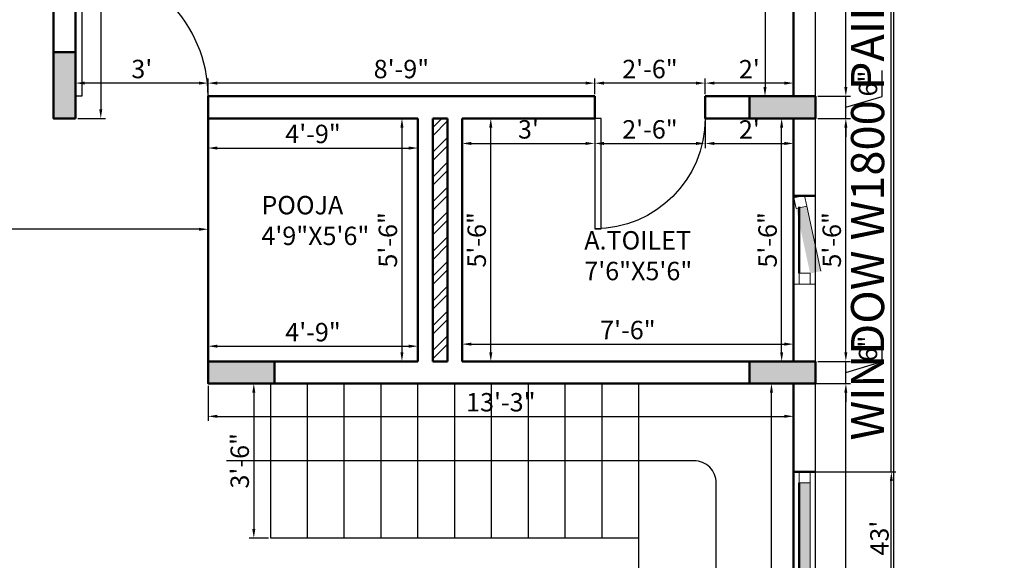
# Model space of a CAD drawing. Units: inches. Extents: x 3064 to 19385, y 846 to 15425.
# Tile 51 of 108: x 6168 to 6436, y 1132 to 1279. Entities that reach past the tile are written whole.
import ezdxf

# ---------------------------------------------------------------- set-up
doc = ezdxf.new("R2010")
doc.units = ezdxf.units.IN
for name, color, linetype, lineweight in [('A-ANNO-DIMS', 2, 'Continuous', 18), ('A-AREA-IDEN', 3, 'Continuous', 18), ('A-COLS', 1, 'Continuous', 35), ('A-DOOR', 3, 'Continuous', 25), ('A-FLOR-STRS', 2, 'Continuous', 25), ('A-FURN-PATT', 252, 'Continuous', 13), ('A-GLAZ', 4, 'Continuous', 18), ('A-WALL', 7, 'Continuous', 50), ('C-PROP', 6, 'Continuous', 25)]:
    doc.layers.add(name, color=color, linetype=linetype, lineweight=lineweight)
doc.styles.get("Standard").update_dxf_attribs({"font": 'arial.ttf'})
doc.dimstyles.new('ISO-25', dxfattribs={"dimtxt": 9, "dimasz": 2.5, "dimexe": 1.25, "dimexo": 0.625, "dimtad": 1, "dimdec": 1, "dimlunit": 3, "dimtxsty": 'Standard', "dimcen": 2.5, "dimadec": 0, "dimazin": 0, "dimtfac": 1, "dimtdec": 1, "dimtmove": 0, "dimatfit": 3, "dimfxl": 1, "dimarcsym": 0})

# ---------------------------------------------------------------- blocks, each defined once
blk = doc.blocks.new('*U3')
for p, q in [((0, 0), (0, -6)), ((36, 0), (36, -6))]:
    blk.add_line(p, q)
blk.add_lwpolyline([(0, 0), (0, 36), (1.75, 36), (1.75, 0)], close=True)
blk.add_arc((0, 0), 36, 0, 90)
blk = doc.blocks.new('*U4')
for p, q in [((0, 0), (0, -6)), ((30, 0), (30, -6))]:
    blk.add_line(p, q)
blk.add_lwpolyline([(0, 0), (0, 30), (1.75, 30), (1.75, 0)], close=True)
blk.add_arc((0, 0), 30, 0, 90)
blk = doc.blocks.new('*D106')
at = {"layer": 'A-ANNO-DIMS', "color": 0, "lineweight": -2, "transparency": 16777216}
for p, q in [((6379.12, 1180.34), (6393.94, 1180.34)), ((6392.69, 984.84), (6392.69, 1177.84)), ((6379.12, 982.34), (6393.94, 982.34))]:
    blk.add_line(p, q, dxfattribs=at)
at = {"layer": 'A-ANNO-DIMS', "color": 0, "transparency": 16777216}
for points in [[(6392.27, 1177.84), (6393.1, 1177.84), (6392.69, 1180.34)], [(6392.27, 984.84), (6393.1, 984.84), (6392.69, 982.34)]]:
    blk.add_solid(points, dxfattribs=at)
at = {"layer": 'Defpoints', "color": 0, "transparency": 16777216}
for p in [(6378.49, 1180.34), (6392.69, 1180.34), (6378.49, 982.34)]:
    blk.add_point(p, dxfattribs=at)
at = {"layer": 'A-ANNO-DIMS', "color": 0, "transparency": 16777216, "insert": (6389.51, 1081.34), "char_height": 5, "attachment_point": 5, "rotation": 90}
blk.add_mtext('16\'-6"', dxfattribs=at)
blk = doc.blocks.new('*D107')
at = {"layer": 'A-ANNO-DIMS', "color": 0, "lineweight": -2, "transparency": 16777216}
for p, q in [((6402.53, 1186.29), (6402.53, 1193.32)), ((6392.69, 1188.84), (6392.69, 1191.34)), ((6385.12, 1186.34), (6393.94, 1186.34)), ((6392.69, 1180.34), (6392.69, 1186.34)), ((6392.69, 1180.34), (6392.69, 1186.34)), ((6392.69, 1183.34), (6402.53, 1186.29)), ((6379.12, 1180.34), (6393.94, 1180.34)), ((6392.69, 1177.84), (6392.69, 1175.34))]:
    blk.add_line(p, q, dxfattribs=at)
at = {"layer": 'A-ANNO-DIMS', "color": 0, "transparency": 16777216}
for points in [[(6392.27, 1188.84), (6393.1, 1188.84), (6392.69, 1186.34)], [(6392.27, 1177.84), (6393.1, 1177.84), (6392.69, 1180.34)]]:
    blk.add_solid(points, dxfattribs=at)
at = {"layer": 'Defpoints', "color": 0, "transparency": 16777216}
for p in [(6384.49, 1186.34), (6392.69, 1186.34), (6378.49, 1180.34)]:
    blk.add_point(p, dxfattribs=at)
at = {"layer": 'A-ANNO-DIMS', "color": 0, "transparency": 16777216, "insert": (6399.35, 1189.81), "char_height": 5, "attachment_point": 5, "rotation": 90}
blk.add_mtext('6"', dxfattribs=at)
blk = doc.blocks.new('*D108')
at = {"layer": 'A-ANNO-DIMS', "color": 0, "lineweight": -2, "transparency": 16777216}
for p, q in [((6385.12, 1252.34), (6393.94, 1252.34)), ((6392.69, 1188.84), (6392.69, 1249.84)), ((6385.12, 1186.34), (6393.94, 1186.34))]:
    blk.add_line(p, q, dxfattribs=at)
at = {"layer": 'A-ANNO-DIMS', "color": 0, "transparency": 16777216}
for points in [[(6392.27, 1249.84), (6393.1, 1249.84), (6392.69, 1252.34)], [(6392.27, 1188.84), (6393.1, 1188.84), (6392.69, 1186.34)]]:
    blk.add_solid(points, dxfattribs=at)
at = {"layer": 'Defpoints', "color": 0, "transparency": 16777216}
for p in [(6384.49, 1252.34), (6392.69, 1252.34), (6384.49, 1186.34)]:
    blk.add_point(p, dxfattribs=at)
at = {"layer": 'A-ANNO-DIMS', "color": 0, "transparency": 16777216, "insert": (6389.51, 1219.34), "char_height": 5, "attachment_point": 5, "rotation": 90}
blk.add_mtext('5\'-6"', dxfattribs=at)
blk = doc.blocks.new('*D109')
at = {"layer": 'A-ANNO-DIMS', "color": 0, "lineweight": -2, "transparency": 16777216}
for p, q in [((6402.53, 1258.29), (6402.53, 1265.32)), ((6392.69, 1260.84), (6392.69, 1263.34)), ((6385.12, 1258.34), (6393.94, 1258.34)), ((6392.69, 1252.34), (6392.69, 1258.34)), ((6392.69, 1252.34), (6392.69, 1258.34)), ((6392.69, 1255.34), (6402.53, 1258.29)), ((6385.12, 1252.34), (6393.94, 1252.34)), ((6392.69, 1249.84), (6392.69, 1247.34))]:
    blk.add_line(p, q, dxfattribs=at)
at = {"layer": 'A-ANNO-DIMS', "color": 0, "transparency": 16777216}
for points in [[(6392.27, 1260.84), (6393.1, 1260.84), (6392.69, 1258.34)], [(6392.27, 1249.84), (6393.1, 1249.84), (6392.69, 1252.34)]]:
    blk.add_solid(points, dxfattribs=at)
at = {"layer": 'Defpoints', "color": 0, "transparency": 16777216}
for p in [(6384.49, 1258.34), (6392.69, 1258.34), (6384.49, 1252.34)]:
    blk.add_point(p, dxfattribs=at)
at = {"layer": 'A-ANNO-DIMS', "color": 0, "transparency": 16777216, "insert": (6399.35, 1261.81), "char_height": 5, "attachment_point": 5, "rotation": 90}
blk.add_mtext('6"', dxfattribs=at)
blk = doc.blocks.new('*D131')
at = {"layer": 'A-ANNO-DIMS', "color": 0, "lineweight": -2, "transparency": 16777216}
for p, q in [((6379.12, 1390.34), (6393.94, 1390.34)), ((6392.69, 1260.84), (6392.69, 1387.84)), ((6385.12, 1258.34), (6393.94, 1258.34))]:
    blk.add_line(p, q, dxfattribs=at)
at = {"layer": 'A-ANNO-DIMS', "color": 0, "transparency": 16777216}
for points in [[(6392.27, 1387.84), (6393.1, 1387.84), (6392.69, 1390.34)], [(6392.27, 1260.84), (6393.1, 1260.84), (6392.69, 1258.34)]]:
    blk.add_solid(points, dxfattribs=at)
at = {"layer": 'Defpoints', "color": 0, "transparency": 16777216}
for p in [(6378.49, 1390.34), (6392.69, 1390.34), (6384.49, 1258.34)]:
    blk.add_point(p, dxfattribs=at)
at = {"layer": 'A-ANNO-DIMS', "color": 0, "transparency": 16777216, "insert": (6389.55, 1324.34), "char_height": 5, "attachment_point": 5, "rotation": 90}
blk.add_mtext("11'", dxfattribs=at)
blk = doc.blocks.new('*D133')
at = {"layer": 'A-ANNO-DIMS', "color": 0, "lineweight": -2, "transparency": 16777216}
for p, q in [((6385.12, 1396.34), (6406.89, 1396.34)), ((6405.64, 1393.84), (6405.64, 882.84)), ((6385.12, 880.34), (6406.89, 880.34))]:
    blk.add_line(p, q, dxfattribs=at)
at = {"layer": 'A-ANNO-DIMS', "color": 0, "transparency": 16777216}
for points in [[(6405.22, 1393.84), (6406.05, 1393.84), (6405.64, 1396.34)], [(6405.22, 882.84), (6406.05, 882.84), (6405.64, 880.34)]]:
    blk.add_solid(points, dxfattribs=at)
at = {"layer": 'Defpoints', "color": 0, "transparency": 16777216}
for p in [(6384.49, 1396.34), (6384.49, 880.34), (6405.64, 880.34)]:
    blk.add_point(p, dxfattribs=at)
at = {"layer": 'A-ANNO-DIMS', "color": 0, "transparency": 16777216, "insert": (6402.46, 1138.34), "char_height": 5, "attachment_point": 5, "rotation": 90}
blk.add_mtext("43'", dxfattribs=at)
blk = doc.blocks.new('*D151')
at = {"layer": 'A-ANNO-DIMS', "color": 0, "lineweight": -2, "transparency": 16777216}
for p, q in [((6377.87, 1390.34), (6369.49, 1390.34)), ((6370.74, 1387.84), (6370.74, 1260.84)), ((6377.87, 1258.34), (6369.49, 1258.34))]:
    blk.add_line(p, q, dxfattribs=at)
at = {"layer": 'A-ANNO-DIMS', "color": 0, "transparency": 16777216}
for points in [[(6370.32, 1387.84), (6371.16, 1387.84), (6370.74, 1390.34)], [(6370.32, 1260.84), (6371.16, 1260.84), (6370.74, 1258.34)]]:
    blk.add_solid(points, dxfattribs=at)
at = {"layer": 'Defpoints', "color": 0, "transparency": 16777216}
for p in [(6378.49, 1390.34), (6370.74, 1258.34), (6378.49, 1258.34)]:
    blk.add_point(p, dxfattribs=at)
at = {"layer": 'A-ANNO-DIMS', "color": 0, "transparency": 16777216, "insert": (6367.61, 1324.34), "char_height": 5, "attachment_point": 5, "rotation": 90}
blk.add_mtext("11'", dxfattribs=at)
blk = doc.blocks.new('*D152')
at = {"layer": 'A-ANNO-DIMS', "color": 0, "lineweight": -2, "transparency": 16777216}
for p, q in [((6354.49, 1258.96), (6354.49, 1263.17)), ((6378.49, 1258.96), (6378.49, 1263.17)), ((6375.99, 1261.92), (6356.99, 1261.92))]:
    blk.add_line(p, q, dxfattribs=at)
at = {"layer": 'A-ANNO-DIMS', "color": 0, "transparency": 16777216}
for points in [[(6356.99, 1262.33), (6356.99, 1261.5), (6354.49, 1261.92)], [(6375.99, 1262.33), (6375.99, 1261.5), (6378.49, 1261.92)]]:
    blk.add_solid(points, dxfattribs=at)
at = {"layer": 'Defpoints', "color": 0, "transparency": 16777216}
for p in [(6354.49, 1261.92), (6354.49, 1258.34), (6378.49, 1258.34)]:
    blk.add_point(p, dxfattribs=at)
at = {"layer": 'A-ANNO-DIMS', "color": 0, "transparency": 16777216, "insert": (6366.49, 1265.05), "char_height": 5, "attachment_point": 5}
blk.add_mtext("2'", dxfattribs=at)
blk = doc.blocks.new('*D153')
at = {"layer": 'A-ANNO-DIMS', "color": 0, "lineweight": -2, "transparency": 16777216}
for p, q in [((6324.49, 1258.96), (6324.49, 1263.17)), ((6354.49, 1258.96), (6354.49, 1263.17)), ((6351.99, 1261.92), (6326.99, 1261.92))]:
    blk.add_line(p, q, dxfattribs=at)
at = {"layer": 'A-ANNO-DIMS', "color": 0, "transparency": 16777216}
for points in [[(6326.99, 1262.33), (6326.99, 1261.5), (6324.49, 1261.92)], [(6351.99, 1262.33), (6351.99, 1261.5), (6354.49, 1261.92)]]:
    blk.add_solid(points, dxfattribs=at)
at = {"layer": 'Defpoints', "color": 0, "transparency": 16777216}
for p in [(6324.49, 1261.92), (6324.49, 1258.34), (6354.49, 1258.34)]:
    blk.add_point(p, dxfattribs=at)
at = {"layer": 'A-ANNO-DIMS', "color": 0, "transparency": 16777216, "insert": (6339.49, 1265.09), "char_height": 5, "attachment_point": 5}
blk.add_mtext('2\'-6"', dxfattribs=at)
blk = doc.blocks.new('*D154')
at = {"layer": 'A-ANNO-DIMS', "color": 0, "lineweight": -2, "transparency": 16777216}
for p, q in [((6219.49, 1258.96), (6219.49, 1263.17)), ((6324.49, 1258.96), (6324.49, 1263.17)), ((6321.99, 1261.92), (6221.99, 1261.92))]:
    blk.add_line(p, q, dxfattribs=at)
at = {"layer": 'A-ANNO-DIMS', "color": 0, "transparency": 16777216}
for points in [[(6221.99, 1262.33), (6221.99, 1261.5), (6219.49, 1261.92)], [(6321.99, 1262.33), (6321.99, 1261.5), (6324.49, 1261.92)]]:
    blk.add_solid(points, dxfattribs=at)
at = {"layer": 'Defpoints', "color": 0, "transparency": 16777216}
for p in [(6219.49, 1261.92), (6219.49, 1258.34), (6324.49, 1258.34)]:
    blk.add_point(p, dxfattribs=at)
at = {"layer": 'A-ANNO-DIMS', "color": 0, "transparency": 16777216, "insert": (6271.99, 1265.09), "char_height": 5, "attachment_point": 5}
blk.add_mtext('8\'-9"', dxfattribs=at)
blk = doc.blocks.new('*D155')
at = {"layer": 'A-ANNO-DIMS', "color": 0, "lineweight": -2, "transparency": 16777216}
for p, q in [((6183.49, 1258.96), (6183.49, 1263.17)), ((6219.49, 1258.96), (6219.49, 1263.17)), ((6216.99, 1261.92), (6185.99, 1261.92))]:
    blk.add_line(p, q, dxfattribs=at)
at = {"layer": 'A-ANNO-DIMS', "color": 0, "transparency": 16777216}
for points in [[(6185.99, 1262.33), (6185.99, 1261.5), (6183.49, 1261.92)], [(6216.99, 1262.33), (6216.99, 1261.5), (6219.49, 1261.92)]]:
    blk.add_solid(points, dxfattribs=at)
at = {"layer": 'Defpoints', "color": 0, "transparency": 16777216}
for p in [(6183.49, 1261.92), (6183.49, 1258.34), (6219.49, 1258.34)]:
    blk.add_point(p, dxfattribs=at)
at = {"layer": 'A-ANNO-DIMS', "color": 0, "transparency": 16777216, "insert": (6201.49, 1265.1), "char_height": 5, "attachment_point": 5}
blk.add_mtext("3'", dxfattribs=at)
blk = doc.blocks.new('*D156')
at = {"layer": 'A-ANNO-DIMS', "color": 0, "lineweight": -2, "transparency": 16777216}
for p, q in [((6184.12, 1390.34), (6191.61, 1390.34)), ((6190.36, 1387.84), (6190.36, 1254.84)), ((6184.12, 1252.34), (6191.61, 1252.34))]:
    blk.add_line(p, q, dxfattribs=at)
at = {"layer": 'A-ANNO-DIMS', "color": 0, "transparency": 16777216}
for points in [[(6189.94, 1387.84), (6190.77, 1387.84), (6190.36, 1390.34)], [(6189.94, 1254.84), (6190.77, 1254.84), (6190.36, 1252.34)]]:
    blk.add_solid(points, dxfattribs=at)
at = {"layer": 'Defpoints', "color": 0, "transparency": 16777216}
for p in [(6183.49, 1390.34), (6183.49, 1252.34), (6190.36, 1252.34)]:
    blk.add_point(p, dxfattribs=at)
at = {"layer": 'A-ANNO-DIMS', "color": 0, "transparency": 16777216, "insert": (6187.18, 1321.34), "char_height": 5, "attachment_point": 5, "rotation": 90}
blk.add_mtext('11\'-6"', dxfattribs=at)
blk = doc.blocks.new('*D157')
at = {"layer": 'A-ANNO-DIMS', "color": 0, "lineweight": -2, "transparency": 16777216}
for p, q in [((6219.49, 1251.71), (6219.49, 1243.03)), ((6276.49, 1251.71), (6276.49, 1243.03)), ((6221.99, 1244.28), (6273.99, 1244.28))]:
    blk.add_line(p, q, dxfattribs=at)
at = {"layer": 'A-ANNO-DIMS', "color": 0, "transparency": 16777216}
for points in [[(6221.99, 1244.7), (6221.99, 1243.86), (6219.49, 1244.28)], [(6273.99, 1244.7), (6273.99, 1243.86), (6276.49, 1244.28)]]:
    blk.add_solid(points, dxfattribs=at)
at = {"layer": 'Defpoints', "color": 0, "transparency": 16777216}
for p in [(6219.49, 1252.34), (6276.49, 1252.34), (6276.49, 1244.28)]:
    blk.add_point(p, dxfattribs=at)
at = {"layer": 'A-ANNO-DIMS', "color": 0, "transparency": 16777216, "insert": (6247.99, 1247.46), "char_height": 5, "attachment_point": 5}
blk.add_mtext('4\'-9"', dxfattribs=at)
blk = doc.blocks.new('*D158')
at = {"layer": 'A-ANNO-DIMS', "color": 0, "lineweight": -2, "transparency": 16777216}
for p, q in [((6275.87, 1252.34), (6270.89, 1252.34)), ((6272.14, 1249.84), (6272.14, 1188.84)), ((6275.87, 1186.34), (6270.89, 1186.34))]:
    blk.add_line(p, q, dxfattribs=at)
at = {"layer": 'A-ANNO-DIMS', "color": 0, "transparency": 16777216}
for points in [[(6271.73, 1249.84), (6272.56, 1249.84), (6272.14, 1252.34)], [(6271.73, 1188.84), (6272.56, 1188.84), (6272.14, 1186.34)]]:
    blk.add_solid(points, dxfattribs=at)
at = {"layer": 'Defpoints', "color": 0, "transparency": 16777216}
for p in [(6276.49, 1252.34), (6272.14, 1186.34), (6276.49, 1186.34)]:
    blk.add_point(p, dxfattribs=at)
at = {"layer": 'A-ANNO-DIMS', "color": 0, "transparency": 16777216, "insert": (6268.97, 1219.34), "char_height": 5, "attachment_point": 5, "rotation": 90}
blk.add_mtext('5\'-6"', dxfattribs=at)
blk = doc.blocks.new('*D159')
at = {"layer": 'A-ANNO-DIMS', "color": 0, "lineweight": -2, "transparency": 16777216}
for p, q in [((6219.49, 1186.96), (6219.49, 1191.72)), ((6221.99, 1190.47), (6273.99, 1190.47)), ((6276.49, 1186.96), (6276.49, 1191.72))]:
    blk.add_line(p, q, dxfattribs=at)
at = {"layer": 'A-ANNO-DIMS', "color": 0, "transparency": 16777216}
for points in [[(6221.99, 1190.88), (6221.99, 1190.05), (6219.49, 1190.47)], [(6273.99, 1190.88), (6273.99, 1190.05), (6276.49, 1190.47)]]:
    blk.add_solid(points, dxfattribs=at)
at = {"layer": 'Defpoints', "color": 0, "transparency": 16777216}
for p in [(6276.49, 1190.47), (6219.49, 1186.34), (6276.49, 1186.34)]:
    blk.add_point(p, dxfattribs=at)
at = {"layer": 'A-ANNO-DIMS', "color": 0, "transparency": 16777216, "insert": (6247.99, 1193.64), "char_height": 5, "attachment_point": 5}
blk.add_mtext('4\'-9"', dxfattribs=at)
blk = doc.blocks.new('*D160')
at = {"layer": 'A-ANNO-DIMS', "color": 0, "lineweight": -2, "transparency": 16777216}
for p, q in [((6288.49, 1186.96), (6288.49, 1192.28)), ((6290.99, 1191.03), (6375.99, 1191.03)), ((6378.49, 1186.96), (6378.49, 1192.28))]:
    blk.add_line(p, q, dxfattribs=at)
at = {"layer": 'A-ANNO-DIMS', "color": 0, "transparency": 16777216}
for points in [[(6290.99, 1191.45), (6290.99, 1190.61), (6288.49, 1191.03)], [(6375.99, 1191.45), (6375.99, 1190.61), (6378.49, 1191.03)]]:
    blk.add_solid(points, dxfattribs=at)
at = {"layer": 'Defpoints', "color": 0, "transparency": 16777216}
for p in [(6378.49, 1191.03), (6288.49, 1186.34), (6378.49, 1186.34)]:
    blk.add_point(p, dxfattribs=at)
at = {"layer": 'A-ANNO-DIMS', "color": 0, "transparency": 16777216, "insert": (6333.49, 1194.21), "char_height": 5, "attachment_point": 5}
blk.add_mtext('7\'-6"', dxfattribs=at)
blk = doc.blocks.new('*D161')
at = {"layer": 'A-ANNO-DIMS', "color": 0, "lineweight": -2, "transparency": 16777216}
for p, q in [((6289.12, 1252.34), (6297.52, 1252.34)), ((6296.27, 1188.84), (6296.27, 1249.84)), ((6289.12, 1186.34), (6297.52, 1186.34))]:
    blk.add_line(p, q, dxfattribs=at)
at = {"layer": 'A-ANNO-DIMS', "color": 0, "transparency": 16777216}
for points in [[(6295.85, 1249.84), (6296.69, 1249.84), (6296.27, 1252.34)], [(6295.85, 1188.84), (6296.69, 1188.84), (6296.27, 1186.34)]]:
    blk.add_solid(points, dxfattribs=at)
at = {"layer": 'Defpoints', "color": 0, "transparency": 16777216}
for p in [(6288.49, 1252.34), (6296.27, 1252.34), (6288.49, 1186.34)]:
    blk.add_point(p, dxfattribs=at)
at = {"layer": 'A-ANNO-DIMS', "color": 0, "transparency": 16777216, "insert": (6293.09, 1219.34), "char_height": 5, "attachment_point": 5, "rotation": 90}
blk.add_mtext('5\'-6"', dxfattribs=at)
blk = doc.blocks.new('*D162')
at = {"layer": 'A-ANNO-DIMS', "color": 0, "lineweight": -2, "transparency": 16777216}
for p, q in [((6288.49, 1251.71), (6288.49, 1244.28)), ((6324.49, 1251.71), (6324.49, 1244.28)), ((6290.99, 1245.53), (6321.99, 1245.53))]:
    blk.add_line(p, q, dxfattribs=at)
at = {"layer": 'A-ANNO-DIMS', "color": 0, "transparency": 16777216}
for points in [[(6290.99, 1245.95), (6290.99, 1245.11), (6288.49, 1245.53)], [(6321.99, 1245.95), (6321.99, 1245.11), (6324.49, 1245.53)]]:
    blk.add_solid(points, dxfattribs=at)
at = {"layer": 'Defpoints', "color": 0, "transparency": 16777216}
for p in [(6288.49, 1252.34), (6324.49, 1252.34), (6324.49, 1245.53)]:
    blk.add_point(p, dxfattribs=at)
at = {"layer": 'A-ANNO-DIMS', "color": 0, "transparency": 16777216, "insert": (6306.49, 1248.71), "char_height": 5, "attachment_point": 5}
blk.add_mtext("3'", dxfattribs=at)
blk = doc.blocks.new('*D163')
at = {"layer": 'A-ANNO-DIMS', "color": 0, "lineweight": -2, "transparency": 16777216}
for p, q in [((6324.49, 1251.71), (6324.49, 1244.28)), ((6354.49, 1251.71), (6354.49, 1244.28)), ((6326.99, 1245.53), (6351.99, 1245.53))]:
    blk.add_line(p, q, dxfattribs=at)
at = {"layer": 'A-ANNO-DIMS', "color": 0, "transparency": 16777216}
for points in [[(6326.99, 1245.95), (6326.99, 1245.11), (6324.49, 1245.53)], [(6351.99, 1245.95), (6351.99, 1245.11), (6354.49, 1245.53)]]:
    blk.add_solid(points, dxfattribs=at)
at = {"layer": 'Defpoints', "color": 0, "transparency": 16777216}
for p in [(6324.49, 1252.34), (6354.49, 1252.34), (6354.49, 1245.53)]:
    blk.add_point(p, dxfattribs=at)
at = {"layer": 'A-ANNO-DIMS', "color": 0, "transparency": 16777216, "insert": (6339.49, 1248.71), "char_height": 5, "attachment_point": 5}
blk.add_mtext('2\'-6"', dxfattribs=at)
blk = doc.blocks.new('*D164')
at = {"layer": 'A-ANNO-DIMS', "color": 0, "lineweight": -2, "transparency": 16777216}
for p, q in [((6354.49, 1251.71), (6354.49, 1244.28)), ((6378.49, 1251.71), (6378.49, 1244.28)), ((6356.99, 1245.53), (6375.99, 1245.53))]:
    blk.add_line(p, q, dxfattribs=at)
at = {"layer": 'A-ANNO-DIMS', "color": 0, "transparency": 16777216}
for points in [[(6356.99, 1245.95), (6356.99, 1245.11), (6354.49, 1245.53)], [(6375.99, 1245.95), (6375.99, 1245.11), (6378.49, 1245.53)]]:
    blk.add_solid(points, dxfattribs=at)
at = {"layer": 'Defpoints', "color": 0, "transparency": 16777216}
for p in [(6354.49, 1252.34), (6378.49, 1252.34), (6378.49, 1245.53)]:
    blk.add_point(p, dxfattribs=at)
at = {"layer": 'A-ANNO-DIMS', "color": 0, "transparency": 16777216, "insert": (6366.49, 1248.67), "char_height": 5, "attachment_point": 5}
blk.add_mtext("2'", dxfattribs=at)
blk = doc.blocks.new('*D165')
at = {"layer": 'A-ANNO-DIMS', "color": 0, "lineweight": -2, "transparency": 16777216}
for p, q in [((6377.87, 1252.34), (6374.01, 1252.34)), ((6375.26, 1188.84), (6375.26, 1249.84)), ((6377.87, 1186.34), (6374.01, 1186.34))]:
    blk.add_line(p, q, dxfattribs=at)
at = {"layer": 'A-ANNO-DIMS', "color": 0, "transparency": 16777216}
for points in [[(6374.84, 1249.84), (6375.67, 1249.84), (6375.26, 1252.34)], [(6374.84, 1188.84), (6375.67, 1188.84), (6375.26, 1186.34)]]:
    blk.add_solid(points, dxfattribs=at)
at = {"layer": 'Defpoints', "color": 0, "transparency": 16777216}
for p in [(6375.26, 1252.34), (6378.49, 1252.34), (6378.49, 1186.34)]:
    blk.add_point(p, dxfattribs=at)
at = {"layer": 'A-ANNO-DIMS', "color": 0, "transparency": 16777216, "insert": (6372.08, 1219.34), "char_height": 5, "attachment_point": 5, "rotation": 90}
blk.add_mtext('5\'-6"', dxfattribs=at)
blk = doc.blocks.new('*D170')
at = {"layer": 'A-ANNO-DIMS', "color": 0, "lineweight": -2, "transparency": 16777216}
for p, q in [((6377.87, 1180.34), (6371.24, 1180.34)), ((6372.49, 984.84), (6372.49, 1177.84)), ((6377.87, 982.34), (6371.24, 982.34))]:
    blk.add_line(p, q, dxfattribs=at)
at = {"layer": 'A-ANNO-DIMS', "color": 0, "transparency": 16777216}
for points in [[(6372.07, 1177.84), (6372.9, 1177.84), (6372.49, 1180.34)], [(6372.07, 984.84), (6372.9, 984.84), (6372.49, 982.34)]]:
    blk.add_solid(points, dxfattribs=at)
at = {"layer": 'Defpoints', "color": 0, "transparency": 16777216}
for p in [(6372.49, 1180.34), (6378.49, 1180.34), (6378.49, 982.34)]:
    blk.add_point(p, dxfattribs=at)
at = {"layer": 'A-ANNO-DIMS', "color": 0, "transparency": 16777216, "insert": (6369.31, 1081.34), "char_height": 5, "attachment_point": 5, "rotation": 90}
blk.add_mtext('16\'-6"', dxfattribs=at)
blk = doc.blocks.new('*D171')
at = {"layer": 'A-ANNO-DIMS', "color": 0, "lineweight": -2, "transparency": 16777216}
for p, q in [((6219.49, 1179.71), (6219.49, 1170.17)), ((6378.49, 1179.71), (6378.49, 1170.17)), ((6221.99, 1171.42), (6375.99, 1171.42))]:
    blk.add_line(p, q, dxfattribs=at)
at = {"layer": 'A-ANNO-DIMS', "color": 0, "transparency": 16777216}
for points in [[(6221.99, 1171.84), (6221.99, 1171.01), (6219.49, 1171.42)], [(6375.99, 1171.84), (6375.99, 1171.01), (6378.49, 1171.42)]]:
    blk.add_solid(points, dxfattribs=at)
at = {"layer": 'Defpoints', "color": 0, "transparency": 16777216}
for p in [(6219.49, 1180.34), (6378.49, 1180.34), (6378.49, 1171.42)]:
    blk.add_point(p, dxfattribs=at)
at = {"layer": 'A-ANNO-DIMS', "color": 0, "transparency": 16777216, "insert": (6298.99, 1174.6), "char_height": 5, "attachment_point": 5}
blk.add_mtext('13\'-3"', dxfattribs=at)
blk = doc.blocks.new('*D172')
at = {"layer": 'A-ANNO-DIMS', "color": 0, "lineweight": -2, "transparency": 16777216}
for p, q in [((6048.49, 1222.85), (6048.49, 1223.48)), ((6216.99, 1222.23), (6050.99, 1222.23)), ((6219.49, 1222.85), (6219.49, 1223.48))]:
    blk.add_line(p, q, dxfattribs=at)
at = {"layer": 'A-ANNO-DIMS', "color": 0, "transparency": 16777216}
for points in [[(6050.99, 1222.64), (6050.99, 1221.81), (6048.49, 1222.23)], [(6216.99, 1222.64), (6216.99, 1221.81), (6219.49, 1222.23)]]:
    blk.add_solid(points, dxfattribs=at)
at = {"layer": 'Defpoints', "color": 0, "transparency": 16777216}
for p in [(6048.49, 1222.23), (6048.49, 1222.23), (6219.49, 1222.23)]:
    blk.add_point(p, dxfattribs=at)
at = {"layer": 'A-ANNO-DIMS', "color": 0, "transparency": 16777216, "insert": (6133.99, 1225.4), "char_height": 5, "attachment_point": 5}
blk.add_mtext('14\'-3"', dxfattribs=at)
blk = doc.blocks.new('*D185')
at = {"layer": 'A-ANNO-DIMS', "color": 0, "lineweight": -2, "transparency": 16777216}
for p, q in [((6235.87, 1180.34), (6230.66, 1180.34)), ((6231.91, 1177.84), (6231.91, 1140.84)), ((6235.87, 1138.34), (6230.66, 1138.34))]:
    blk.add_line(p, q, dxfattribs=at)
at = {"layer": 'A-ANNO-DIMS', "color": 0, "transparency": 16777216}
for points in [[(6231.5, 1177.84), (6232.33, 1177.84), (6231.91, 1180.34)], [(6231.5, 1140.84), (6232.33, 1140.84), (6231.91, 1138.34)]]:
    blk.add_solid(points, dxfattribs=at)
at = {"layer": 'Defpoints', "color": 0, "transparency": 16777216}
for p in [(6236.49, 1180.34), (6231.91, 1138.34), (6236.49, 1138.34)]:
    blk.add_point(p, dxfattribs=at)
at = {"layer": 'A-ANNO-DIMS', "color": 0, "transparency": 16777216, "insert": (6228.73, 1159.34), "char_height": 5, "attachment_point": 5, "rotation": 90}
blk.add_mtext('3\'-6"', dxfattribs=at)
blk = doc.blocks.new('WIN-600')
h = blk.add_hatch(color=256)
h.dxf.hatch_style = 1
h.paths.add_polyline_path([(3, 18), (0, 18), (0, 0), (3, 0)])
blk.add_line((3, 18), (3, 0))
blk.add_lwpolyline([(3, 18), (0, 18), (0, 21), (3, 21)], close=True)
blk = doc.blocks.new('WIN-1800-PAIR')
h = blk.add_hatch(color=256)
h.dxf.hatch_style = 1
h.paths.add_polyline_path([(0, 0), (3, 0), (3, 70.5), (0, 70.5)])
h.paths.add_polyline_path([(3, 144), (0, 144), (0, 73.5), (3, 73.5)])
blk.add_line((3, 144), (3, 73.5))
blk.add_lwpolyline([(3, 144), (0, 144), (0, 147), (3, 147)], close=True)
blk = doc.blocks.new('*D445')
at = {"layer": 'A-ANNO-DIMS', "color": 0, "lineweight": -2, "transparency": 16777216}
for p, q in [((6405.04, 1156.34), (6405.04, 1357.14)), ((6383.62, 1156.34), (6406.29, 1156.34)), ((6405.04, 1011.84), (6405.04, 1153.84)), ((6383.62, 1009.34), (6406.29, 1009.34))]:
    blk.add_line(p, q, dxfattribs=at)
at = {"layer": 'A-ANNO-DIMS', "color": 0, "transparency": 16777216}
for points in [[(6404.63, 1153.84), (6405.46, 1153.84), (6405.04, 1156.34)], [(6404.63, 1011.84), (6405.46, 1011.84), (6405.04, 1009.34)]]:
    blk.add_solid(points, dxfattribs=at)
at = {"layer": 'Defpoints', "color": 0, "transparency": 16777216}
for p in [(6382.99, 1156.34), (6405.04, 1156.34), (6382.99, 1009.34)]:
    blk.add_point(p, dxfattribs=at)
at = {"layer": 'A-ANNO-DIMS', "color": 0, "transparency": 16777216, "insert": (6399.76, 1257.99), "char_height": 9, "attachment_point": 5, "rotation": 90}
blk.add_mtext('WINDOW W1800 PAIR 12\'-3" TYP.', dxfattribs=at)

msp = doc.modelspace()

# ---------------------------------------------------------------- hatches: boundary and pattern name
at = {"layer": 'A-COLS'}
h = msp.add_hatch(color=256, dxfattribs=at)
h.dxf.hatch_style = 1
h.paths.add_polyline_path([(6177.49, 1252.34), (6183.49, 1252.34), (6183.49, 1270.34), (6177.49, 1270.34)])
h = msp.add_hatch(color=256, dxfattribs=at)
h.dxf.hatch_style = 1
h.paths.add_polyline_path([(6384.49, 1252.34), (6384.49, 1258.34), (6366.49, 1258.34), (6366.49, 1252.34)])
h = msp.add_hatch(color=256, dxfattribs=at)
h.dxf.hatch_style = 1
h.paths.add_polyline_path([(6237.49, 1180.34), (6237.49, 1186.34), (6219.49, 1186.34), (6219.49, 1180.34)])
h = msp.add_hatch(color=256, dxfattribs=at)
h.dxf.hatch_style = 1
h.paths.add_polyline_path([(6384.49, 1180.34), (6384.49, 1186.34), (6366.49, 1186.34), (6366.49, 1180.34)])
at = {"layer": 'A-FURN-PATT'}
h = msp.add_hatch(dxfattribs=at)
h.set_pattern_fill('ANSI32', color=256, scale=0.5)
h.set_pattern_definition([(45, (726.825, 0), (-3.367596, 3.367596), []), (45, (729.07, 0), (-3.367596, 3.367596), [])])
h.paths.add_polyline_path([(6280.49, 1186.34), (6284.49, 1186.34), (6284.49, 1252.34), (6280.49, 1252.34)])

# ---------------------------------------------------------------- linework, layer by layer
at = {"layer": 'A-FLOR-STRS'}
for p, q in [((6236.49, 1138.34), (6236.49, 1180.34)), ((6246.49, 1138.34), (6246.49, 1180.34)), ((6256.49, 1138.34), (6256.49, 1180.34)), ((6266.49, 1138.34), (6266.49, 1180.34)), ((6276.49, 1138.34), (6276.49, 1180.34)), ((6286.49, 1138.34), (6286.49, 1180.34)), ((6296.49, 1138.34), (6296.49, 1180.34)), ((6306.49, 1138.34), (6306.49, 1180.34)), ((6316.49, 1138.34), (6316.49, 1180.34)), ((6326.49, 1138.34), (6326.49, 1180.34)), ((6336.49, 1024.34), (6336.49, 1180.34)), ((6336.49, 1138.34), (6236.49, 1138.34))]:
    msp.add_line(p, q, dxfattribs=at)
msp.add_lwpolyline([(6243.98, 1003.34), (6351.49, 1003.34, 0.414214), (6357.49, 1009.34), (6357.49, 1153.34, 0.414214), (6351.49, 1159.34), (6224.49, 1159.34)], format="xyb", dxfattribs=at)
at = {"layer": 'A-GLAZ'}
msp.add_line((6378.49, 1207.34), (6384.49, 1207.34), dxfattribs=at)
msp.add_lwpolyline([(6382.99, 1207.34), (6379.99, 1207.34), (6379.99, 1210.34), (6382.99, 1210.34)], close=True, dxfattribs=at)
at = {"layer": 'A-WALL'}
for p, q in [((6177.49, 1390.34), (6177.49, 1252.34)), ((6183.49, 1390.34), (6183.49, 1252.34)), ((6378.49, 1258.34), (6378.49, 1390.34)), ((6324.49, 1258.34), (6219.49, 1258.34)), ((6219.49, 1258.34), (6219.49, 1180.34)), ((6324.49, 1252.34), (6324.49, 1258.34)), ((6354.49, 1252.34), (6354.49, 1258.34)), ((6378.49, 1258.34), (6354.49, 1258.34)), ((6183.49, 1252.34), (6177.49, 1252.34)), ((6276.49, 1252.34), (6219.49, 1252.34)), ((6276.49, 1252.34), (6276.49, 1186.34)), ((6284.49, 1252.34), (6280.49, 1252.34)), ((6280.49, 1252.34), (6280.49, 1186.34)), ((6284.49, 1186.34), (6284.49, 1252.34)), ((6288.49, 1186.34), (6288.49, 1252.34)), ((6324.49, 1252.34), (6288.49, 1252.34)), ((6378.49, 1252.34), (6354.49, 1252.34)), ((6378.49, 1186.34), (6378.49, 1252.34)), ((6378.49, 1231.34), (6384.49, 1231.34)), ((6379.99, 1228.34), (6379.99, 1210.34)), ((6276.49, 1186.34), (6219.49, 1186.34)), ((6284.49, 1186.34), (6280.49, 1186.34)), ((6378.49, 1186.34), (6288.49, 1186.34)), ((6378.49, 1180.34), (6219.49, 1180.34)), ((6378.49, 982.34), (6378.49, 1180.34)), ((6384.49, 1156.34), (6378.49, 1156.34)), ((6379.99, 1153.34), (6379.99, 1082.84))]:
    msp.add_line(p, q, dxfattribs=at)
for points in [[(6183.49, 1252.34), (6183.49, 1270.34), (6177.49, 1270.34), (6177.49, 1252.34)], [(6384.49, 1258.34), (6366.49, 1258.34), (6366.49, 1252.34), (6384.49, 1252.34)], [(6237.49, 1186.34), (6219.49, 1186.34), (6219.49, 1180.34), (6237.49, 1180.34)], [(6384.49, 1186.34), (6366.49, 1186.34), (6366.49, 1180.34), (6384.49, 1180.34)]]:
    msp.add_lwpolyline(points, close=True, dxfattribs=at)
at = {"layer": 'C-PROP'}
msp.add_line((6384.49, 880.34), (6384.49, 1396.34), dxfattribs=at)

# ---------------------------------------------------------------- block references
at = {"layer": 'A-DOOR'}
msp.add_blockref('*U3', (6183.49, 1258.34), dxfattribs=at)
at = {"layer": 'A-DOOR', "xscale": -1, "rotation": 180}
msp.add_blockref('*U4', (6324.49, 1252.34), dxfattribs=at)
at = {"layer": 'A-GLAZ', "rotation": 12.21571913412712}
msp.add_blockref('WIN-600', (6383, 1210.23), dxfattribs=at)
at = {"layer": 'A-GLAZ'}
msp.add_blockref('WIN-1800-PAIR', (6379.99, 1009.34), dxfattribs=at)

# ---------------------------------------------------------------- texts
at = {"layer": 'A-AREA-IDEN', "char_height": 5, "attachment_point": 1}
for s, insert in [('POOJA\\P4\'9"X5\'6"', (6233.97, 1231.27)), ('A.TOILET\\P7\'6"X5\'6"', (6321.66, 1221.72))]:
    msp.add_mtext_dynamic_manual_height_columns(s, width=67.5924, gutter_width=12.5, heights=[0], dxfattribs=dict(at, insert=insert))

# ---------------------------------------------------------------- dimensions: what is measured, and where the dimension line sits
at = {"layer": 'A-ANNO-DIMS'}
for base, p1, p2, override, picture, middle in [((6405.64, 880.34), (6384.49, 1396.34), (6384.49, 880.34), {"dimtxt": 5, "dimclrd": 0, "dimclre": 0, "dimclrt": 0}, '*D133', (6402.46, 1138.34)), ((6190.36, 1252.34), (6183.49, 1390.34), (6183.49, 1252.34), {"dimtxt": 5, "dimclrd": 0, "dimclre": 0, "dimclrt": 0}, '*D156', (6187.18, 1321.34)), ((6370.74, 1258.34), (6378.49, 1390.34), (6378.49, 1258.34), {"dimtxt": 5, "dimclrd": 0, "dimclre": 0, "dimclrt": 0}, '*D151', (6367.61, 1324.34)), ((6392.69, 1390.34), (6384.49, 1258.34), (6378.49, 1390.34), {"dimtxt": 5, "dimclrd": 0, "dimclre": 0, "dimclrt": 0, "dimtmove": 1}, '*D131', (6389.55, 1324.34)), ((6392.69, 1258.34), (6384.49, 1252.34), (6384.49, 1258.34), {"dimtxt": 5, "dimclrd": 0, "dimclre": 0, "dimclrt": 0, "dimtmove": 1}, '*D109', (6399.35, 1258.92)), ((6272.14, 1186.34), (6276.49, 1252.34), (6276.49, 1186.34), {"dimtxt": 5, "dimclrd": 0, "dimclre": 0, "dimclrt": 0}, '*D158', (6268.97, 1219.34)), ((6296.27, 1252.34), (6288.49, 1186.34), (6288.49, 1252.34), {"dimtxt": 5, "dimclrd": 0, "dimclre": 0, "dimclrt": 0}, '*D161', (6293.09, 1219.34)), ((6375.26, 1252.34), (6378.49, 1186.34), (6378.49, 1252.34), {"dimtxt": 5, "dimclrd": 0, "dimclre": 0, "dimclrt": 0}, '*D165', (6372.08, 1219.34)), ((6392.69, 1252.34), (6384.49, 1186.34), (6384.49, 1252.34), {"dimtxt": 5, "dimclrd": 0, "dimclre": 0, "dimclrt": 0, "dimtmove": 1}, '*D108', (6389.51, 1219.34)), ((6392.69, 1186.34), (6378.49, 1180.34), (6384.49, 1186.34), {"dimtxt": 5, "dimclrd": 0, "dimclre": 0, "dimclrt": 0, "dimtmove": 1}, '*D107', (6399.35, 1186.92)), ((6231.91, 1138.34), (6236.49, 1180.34), (6236.49, 1138.34), {"dimtxt": 5, "dimclrd": 0, "dimclre": 0, "dimclrt": 0}, '*D185', (6228.73, 1159.34)), ((6372.49, 1180.34), (6378.49, 982.34), (6378.49, 1180.34), {"dimtxt": 5, "dimclrd": 0, "dimclre": 0, "dimclrt": 0}, '*D170', (6369.31, 1081.34)), ((6392.69, 1180.34), (6378.49, 982.34), (6378.49, 1180.34), {"dimtxt": 5, "dimclrd": 0, "dimclre": 0, "dimclrt": 0, "dimtmove": 1}, '*D106', (6389.51, 1081.34))]:
    dim = msp.add_linear_dim(base=base, p1=p1, p2=p2, angle=90, dimstyle='ISO-25', override=override, dxfattribs=at)
    dim.commit()
    dim.dimension.update_dxf_attribs({"geometry": picture, "text_midpoint": middle})
dim = msp.add_linear_dim(base=(6405.04, 1156.34), p1=(6382.99, 1009.34), p2=(6382.99, 1156.34), angle=90, text='WINDOW W1800 PAIR <> TYP.', dimstyle='ISO-25', override={"dimdec": 1, "dimrnd": 0, "dimzin": 1, "dimlunit": 4, "dimfrac": 2}, dxfattribs=at)
dim.commit()
dim.dimension.update_dxf_attribs({"geometry": '*D445', "text_midpoint": (6399.76, 1257.99)})
for base, p1, p2, override, picture, middle in [((6183.49, 1261.92), (6219.49, 1258.34), (6183.49, 1258.34), {"dimtxt": 5, "dimclrd": 0, "dimclre": 0, "dimclrt": 0, "dimtmove": 1}, '*D155', (6201.49, 1265.1)), ((6219.49, 1261.92), (6324.49, 1258.34), (6219.49, 1258.34), {"dimtxt": 5, "dimclrd": 0, "dimclre": 0, "dimclrt": 0, "dimtmove": 1}, '*D154', (6271.99, 1265.09)), ((6324.49, 1261.92), (6354.49, 1258.34), (6324.49, 1258.34), {"dimtxt": 5, "dimclrd": 0, "dimclre": 0, "dimclrt": 0, "dimtmove": 1}, '*D153', (6339.49, 1265.09)), ((6354.49, 1261.92), (6378.49, 1258.34), (6354.49, 1258.34), {"dimtxt": 5, "dimclrd": 0, "dimclre": 0, "dimclrt": 0}, '*D152', (6366.49, 1265.05)), ((6276.49, 1244.28), (6219.49, 1252.34), (6276.49, 1252.34), {"dimtxt": 5, "dimclrd": 0, "dimclre": 0, "dimclrt": 0}, '*D157', (6247.99, 1247.46)), ((6324.49, 1245.53), (6288.49, 1252.34), (6324.49, 1252.34), {"dimtxt": 5, "dimclrd": 0, "dimclre": 0, "dimclrt": 0}, '*D162', (6306.49, 1248.71)), ((6354.49, 1245.53), (6324.49, 1252.34), (6354.49, 1252.34), {"dimtxt": 5, "dimclrd": 0, "dimclre": 0, "dimclrt": 0, "dimtmove": 1}, '*D163', (6339.49, 1248.71)), ((6378.49, 1245.53), (6354.49, 1252.34), (6378.49, 1252.34), {"dimtxt": 5, "dimclrd": 0, "dimclre": 0, "dimclrt": 0, "dimtmove": 1}, '*D164', (6366.49, 1248.67)), ((6048.49, 1222.23), (6219.49, 1222.23), (6048.49, 1222.23), {"dimtxt": 5, "dimclrd": 0, "dimclre": 0, "dimclrt": 0}, '*D172', (6133.99, 1225.4)), ((6276.49, 1190.47), (6219.49, 1186.34), (6276.49, 1186.34), {"dimtxt": 5, "dimclrd": 0, "dimclre": 0, "dimclrt": 0}, '*D159', (6247.99, 1193.64)), ((6378.49, 1191.03), (6288.49, 1186.34), (6378.49, 1186.34), {"dimtxt": 5, "dimclrd": 0, "dimclre": 0, "dimclrt": 0}, '*D160', (6333.49, 1194.21)), ((6378.49, 1171.42), (6219.49, 1180.34), (6378.49, 1180.34), {"dimtxt": 5, "dimclrd": 0, "dimclre": 0, "dimclrt": 0}, '*D171', (6298.99, 1174.6))]:
    dim = msp.add_linear_dim(base=base, p1=p1, p2=p2, dimstyle='ISO-25', override=override, dxfattribs=at)
    dim.commit()
    dim.dimension.update_dxf_attribs({"geometry": picture, "text_midpoint": middle})

doc.saveas('drawing.dxf')
